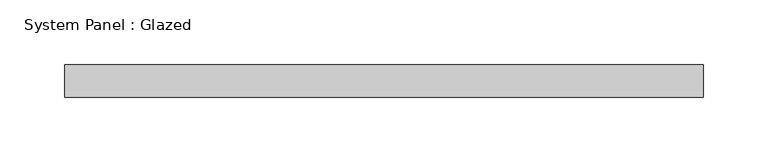
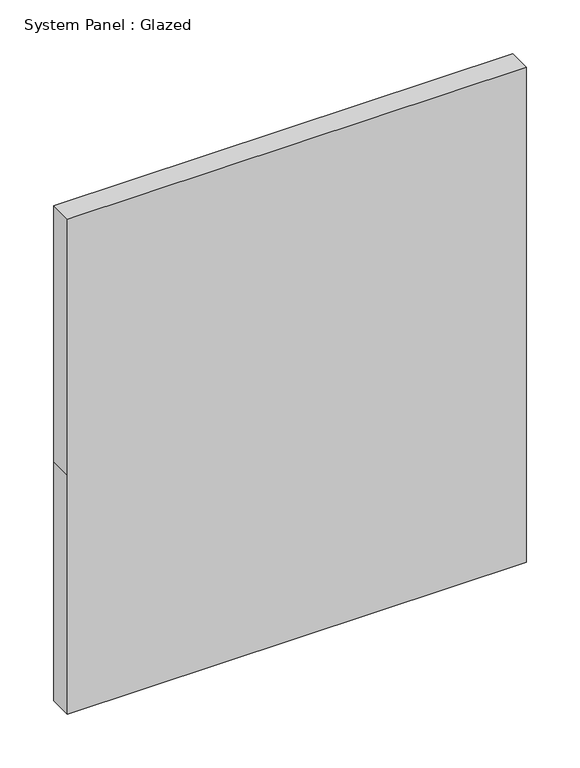
"""IFC4 building model written with IfcOpenShell, lengths in millimetres: plate geometry, System Panel : Glazed."""

from ifc_helpers import new_model, si_unit, frame, origin, place, context, project, spatial, polyline, outline, extrude, source, transform, mapped, element, save


def system_panel_glazed_080879d4(model_context):
    return source(origin(), model_context, "Body", "SweptSolid", [
        extrude(outline(polyline([(0.0, -247.65), (0.0, 247.65), (273.05, 247.65), (565.15, 247.65), (565.15, -247.65), (273.05, -247.65), (0.0, -247.65)])), frame((0.0, 19.05, 0.0), z_axis=(0.0, 1.0, 0.0), x_axis=(0.0, 0.0, 1.0)), (0.0, 0.0, 1.0), 25.4),
    ])


if __name__ == "__main__":
    model = new_model("IFC4")
    model_context = context("Model", 3, world=origin())
    ifc_project = project(units=[si_unit("LENGTHUNIT", "METRE", prefix="MILLI")], contexts=[model_context])
    site = spatial("IfcSite", under=ifc_project)
    building = spatial("IfcBuilding", under=site)
    placement = place(None, origin())
    system_panel_glazed_shape = system_panel_glazed_080879d4(model_context)
    element("IfcPlate", 1, ObjectType="System Panel : Glazed", at=placement, inside=building, context=model_context, shape_type="MappedRepresentation", body=[
        mapped(system_panel_glazed_shape, transform((0.0, 0.0, 0.0), x_axis=(1.0, 0.0, 0.0), y_axis=(0.0, 1.0, 0.0), z_axis=(0.0, 0.0, 1.0))),
    ])
    save(model, "model.ifc")

# Revit data of these elements
# Type "System Panel : Glazed"
#   Construction Type Id = "GSP4R"
#   Analytic Construction = "1/8 in Pilkington single glazing"
#   Visual Light Transmittance = 0.9
#   Solar Heat Gain Coefficient = 0.86
#   Heat Transfer Coefficient (U) = 1.18115 BTU/(h·ft²·°F)
#   Define Thermal Properties by = 1
# Element 1 (IfcPlate, "System Panel : Glazed")
#   Materials on its faces: "Glass"
# Materials
#   "Glass": class "Glass", colour RGB 0 128 192, transparency 0.75, Description = "Soda Lime Glass", Cost = 0
